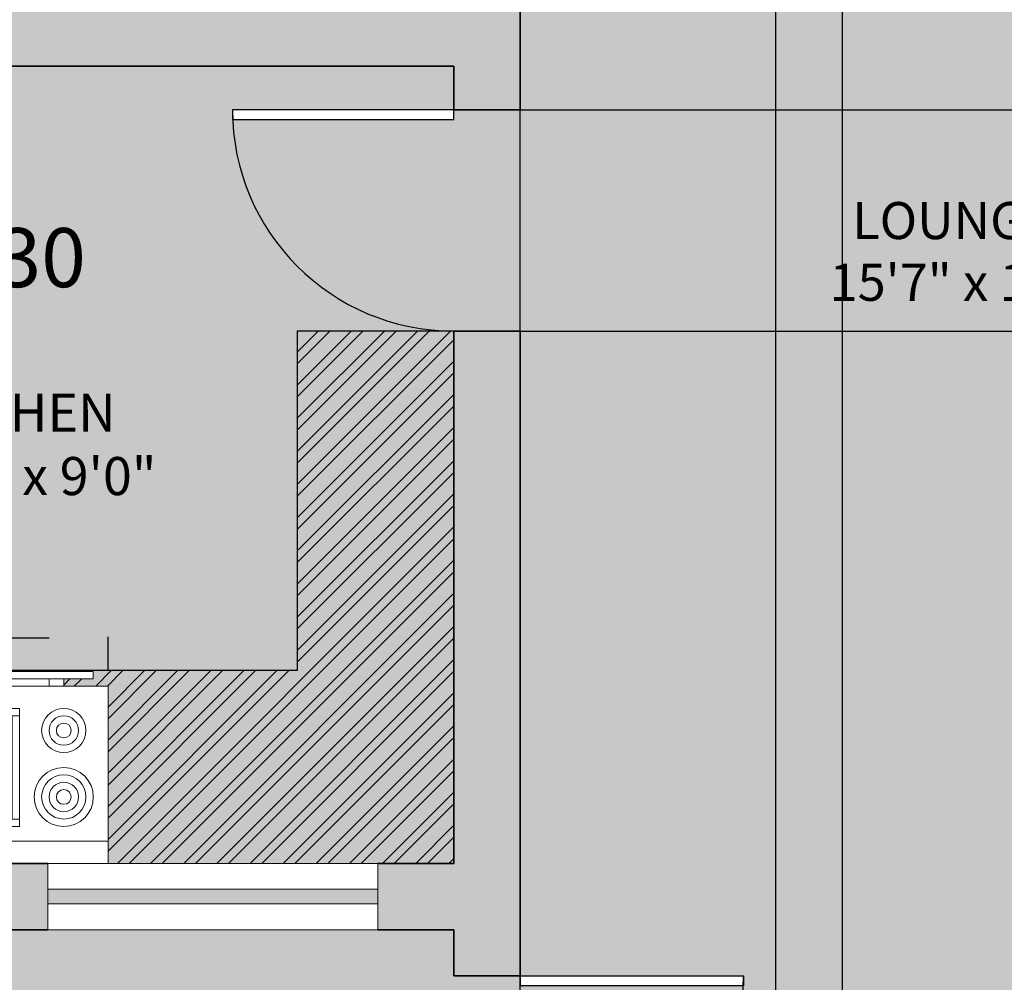
# Model space of a CAD drawing. Units: inches. Extents: x 389 to 971, y 148 to 870.
# Tile 9 of 14: x 537 to 670, y 428 to 558. Entities that reach past the tile are written whole.
import ezdxf

# ---------------------------------------------------------------- set-up
doc = ezdxf.new("R2010")
doc.units = ezdxf.units.IN
doc.header["$MEASUREMENT"] = 0
for name, color, linetype, lineweight in [('A-ANNO-DIMS', 2, 'Continuous', 18), ('A-AREA-IDEN', 7, 'Continuous', 18), ('A-CSWK-PATT', 9, 'Continuous', 13), ('A-DOOR', 4, 'Continuous', 25), ('A-EQPM', 8, 'Continuous', 18), ('A-FLOR-BASE-PATT', 8, 'Continuous', 13), ('A-FLOR-CSWK', 7, 'Continuous', 25), ('A-GLAZ', 4, 'Continuous', 18), ('A-WALL', 7, 'Continuous', 35), ('L-GRND-BASE-PATT', 8, 'Continuous', 13)]:
    doc.layers.add(name, color=color, linetype=linetype, lineweight=lineweight)
for name, color, linetype, lineweight, true_color in [('A-CSWK-BASE-PATT', 18, 'Continuous', 13, 0x000000), ('A-GLAZ-PATT', 251, 'Continuous', 13, 0x6d5f6c), ('A-WALL-PATT', 18, 'Continuous', 13, 0x000000), ('L-GRND-PATT', 39, 'Continuous', 13, 0x603913)]:
    doc.layers.add(name, color=color, linetype=linetype, lineweight=lineweight, true_color=true_color)
doc.styles.get("Standard").update_dxf_attribs({"font": 'arial.ttf'})
doc.dimstyles.get("Standard").update_dxf_attribs({"dimtxt": 8, "dimasz": 8, "dimexe": 0.18, "dimexo": 0.0625, "dimgap": 0.09, "dimtad": 0, "dimtih": 1, "dimtoh": 1, "dimdec": 0, "dimzin": 0, "dimdsep": 46, "dimlunit": 3, "dimtxsty": 'Standard', "dimcen": 0.09, "dimadec": 0, "dimazin": 0, "dimtfac": 1, "dimtdec": 0, "dimtofl": 0, "dimtmove": 0, "dimatfit": 3, "dimfxl": 1, "dimtolj": 1, "dimtzin": 0, "dimarcsym": 0})
pattern_1 = [(45, (0, 0), (-2.245064, 2.245064), []), (45, (0, 1.5875), (-2.245064, 2.245064), [])]

# ---------------------------------------------------------------- blocks, each defined once
blk = doc.blocks.new('*U2')
for p, q in [((0, 0), (0, -6)), ((40, 0), (40, -6))]:
    blk.add_line(p, q)
blk.add_lwpolyline([(0, 0), (0, 40), (1.75, 40), (1.75, 0)], close=True)
blk.add_arc((0, 0), 40, 0, 90)
blk = doc.blocks.new('*U3')
for p, q in [((0, 0), (0, -6)), ((-40, 0), (-40, -6))]:
    blk.add_line(p, q)
blk.add_lwpolyline([(0, 0), (0, 40), (-1.75, 40), (-1.75, 0)], close=True)
blk.add_arc((0, 0), 40, 90, 180)
blk = doc.blocks.new('Range-Oven - 30 in top')
for p, q in [((0, -3), (30, -3)), ((12, -6), (18, -6)), ((13, -20), (13, -6)), ((14, -6), (14, -20)), ((15, -20), (15, -6)), ((16, -6), (16, -20)), ((17, -20), (17, -6)), ((18, -20), (12, -20)), ((6, -24), (6, -25)), ((8, -25), (8, -24)), ((22, -25), (22, -24)), ((24, -24), (24, -25))]:
    blk.add_line(p, q)
for points in [[(0, -24), (0, 0), (30, 0), (30, -24)], [(12, -21), (12, -5), (18, -5), (18, -21)], [(2, -26), (2, -25), (28, -25), (28, -26)]]:
    blk.add_lwpolyline(points, close=True)
for centre, radius in [((6, -9), 4), ((6, -9), 3), ((24, -9), 3), ((6, -9), 2), ((6, -9), 1), ((24, -9), 2), ((24, -9), 1), ((24, -18), 4), ((6, -18), 3), ((6, -18), 2), ((24, -18), 3), ((24, -18), 2), ((6, -18), 1), ((24, -18), 1)]:
    blk.add_circle(centre, radius)
blk = doc.blocks.new('*D32')
at = {"layer": 'A-ANNO-DIMS', "color": 0, "lineweight": -2, "transparency": 16777216}
for p, q in [((518.55, 474.14), (510.55, 474.14)), ((518.55, 469.71), (518.55, 474.32)), ((540.55, 474.14), (526.55, 474.14)), ((548.55, 469.71), (548.55, 474.32))]:
    blk.add_line(p, q, dxfattribs=at)
at = {"layer": 'A-ANNO-DIMS', "color": 0, "transparency": 16777216}
for points in [[(526.55, 475.48), (526.55, 472.81), (518.55, 474.14)], [(540.55, 475.48), (540.55, 472.81), (548.55, 474.14)]]:
    blk.add_solid(points, dxfattribs=at)
at = {"layer": 'Defpoints', "color": 0, "transparency": 16777216}
for p in [(518.55, 474.14), (518.55, 469.64), (548.55, 469.64)]:
    blk.add_point(p, dxfattribs=at)
at = {"layer": 'A-ANNO-DIMS', "color": 0, "transparency": 16777216, "insert": (483.53, 474.14), "char_height": 8, "attachment_point": 5}
blk.add_mtext('\\A1;RANGE 30', dxfattribs=at)
blk = doc.blocks.new('*D34')
at = {"layer": 'A-ANNO-DIMS', "color": 0, "lineweight": -2, "transparency": 16777216}
for p, q in [((497.28, 540.7), (501.9, 540.7)), ((501.72, 532.7), (501.72, 529.93)), ((501.72, 518.7), (501.72, 521.47)), ((497.28, 510.7), (501.9, 510.7))]:
    blk.add_line(p, q, dxfattribs=at)
at = {"layer": 'A-ANNO-DIMS', "color": 0, "transparency": 16777216}
for points in [[(500.38, 532.7), (503.05, 532.7), (501.72, 540.7)], [(500.38, 518.7), (503.05, 518.7), (501.72, 510.7)]]:
    blk.add_solid(points, dxfattribs=at)
at = {"layer": 'Defpoints', "color": 0, "transparency": 16777216}
for p in [(497.22, 540.7), (501.72, 540.7), (497.22, 510.7)]:
    blk.add_point(p, dxfattribs=at)
at = {"layer": 'A-ANNO-DIMS', "color": 0, "transparency": 16777216, "insert": (501.72, 525.7), "char_height": 8, "attachment_point": 5}
blk.add_mtext('\\A1;KITCHEN SINK 30', dxfattribs=at)
blk = doc.blocks.new('*D48')
at = {"layer": 'A-ANNO-DIMS', "color": 0, "lineweight": -2, "transparency": 16777216}
for p, q in [((595.45, 545.73), (878.72, 545.73)), ((878.54, 537.73), (878.54, 534.91)), ((878.54, 523.73), (878.54, 526.55)), ((595.45, 515.73), (878.72, 515.73))]:
    blk.add_line(p, q, dxfattribs=at)
at = {"layer": 'A-ANNO-DIMS', "color": 0, "transparency": 16777216}
for points in [[(877.21, 537.73), (879.87, 537.73), (878.54, 545.73)], [(877.21, 523.73), (879.87, 523.73), (878.54, 515.73)]]:
    blk.add_solid(points, dxfattribs=at)
at = {"layer": 'Defpoints', "color": 0, "transparency": 16777216}
for p in [(595.39, 545.73), (878.54, 545.73), (595.39, 515.73)]:
    blk.add_point(p, dxfattribs=at)
at = {"layer": 'A-ANNO-DIMS', "color": 0, "transparency": 16777216, "insert": (878.54, 530.73), "char_height": 8, "attachment_point": 5}
blk.add_mtext('\\A1;30.005', dxfattribs=at)
blk = doc.blocks.new('*D51')
at = {"layer": 'A-ANNO-DIMS', "color": 0, "lineweight": -2, "transparency": 16777216}
for p, q in [((596.39, 864.97), (588.39, 864.97)), ((604.39, 354.78), (604.39, 865.15)), ((639.03, 354.78), (639.03, 865.15)), ((647.03, 864.97), (655.03, 864.97))]:
    blk.add_line(p, q, dxfattribs=at)
at = {"layer": 'A-ANNO-DIMS', "color": 0, "transparency": 16777216}
for points in [[(596.39, 866.3), (596.39, 863.64), (604.39, 864.97)], [(647.03, 866.3), (647.03, 863.64), (639.03, 864.97)]]:
    blk.add_solid(points, dxfattribs=at)
at = {"layer": 'Defpoints', "color": 0, "transparency": 16777216}
for p in [(639.03, 864.97), (604.39, 354.72), (639.03, 354.72)]:
    blk.add_point(p, dxfattribs=at)
at = {"layer": 'A-ANNO-DIMS', "color": 0, "transparency": 16777216, "insert": (621.71, 864.97), "char_height": 8, "attachment_point": 5}
blk.add_mtext('\\A1;34.64', dxfattribs=at)
blk = doc.blocks.new('*D52')
at = {"layer": 'A-ANNO-DIMS', "color": 0, "lineweight": -2, "transparency": 16777216}
for p, q in [((640.06, 864.97), (632.06, 864.97)), ((648.06, 388.98), (648.06, 865.15)), ((690.22, 388.98), (690.22, 865.15)), ((698.22, 864.97), (706.22, 864.97))]:
    blk.add_line(p, q, dxfattribs=at)
at = {"layer": 'A-ANNO-DIMS', "color": 0, "transparency": 16777216}
for points in [[(640.06, 866.3), (640.06, 863.64), (648.06, 864.97)], [(698.22, 866.3), (698.22, 863.64), (690.22, 864.97)]]:
    blk.add_solid(points, dxfattribs=at)
at = {"layer": 'Defpoints', "color": 0, "transparency": 16777216}
for p in [(690.22, 864.97), (648.06, 388.92), (690.22, 388.92)]:
    blk.add_point(p, dxfattribs=at)
at = {"layer": 'A-ANNO-DIMS', "color": 0, "transparency": 16777216, "insert": (669.14, 864.97), "char_height": 8, "attachment_point": 5}
blk.add_mtext('\\A1;42.155', dxfattribs=at)

msp = doc.modelspace()

# ---------------------------------------------------------------- hatches: boundary and pattern name
at = {"layer": 'A-CSWK-BASE-PATT'}
h = msp.add_hatch(color=256, dxfattribs=at)
h.dxf.hatch_style = 1
h.paths.add_polyline_path([(546.5523, 469.7503), (546.5523, 468.6445), (542.5523, 468.6445), (542.5523, 467.6445), (548.5523, 467.6445), (548.5523, 443.6445), (585.0791, 443.6445), (595.387, 443.6445), (595.387, 515.7271), (574.1873, 515.7271), (574.1873, 469.7503)])
at = {"layer": 'A-CSWK-PATT'}
h = msp.add_hatch(dxfattribs=at)
h.set_pattern_fill('STEEL', color=256)
h.set_pattern_definition(pattern_1)
h.paths.add_polyline_path([(477.216, 551.6445), (477.216, 543.0462), (477.216, 508.3496), (477.216, 490.1255), (477.216, 452.1978), (477.216, 443.6445), (488.4095, 443.6445), (526.7125, 443.6445), (540.3922, 443.6445), (585.0791, 443.6445), (595.387, 443.6445), (595.387, 515.7271), (574.1873, 515.7271), (574.1873, 469.7503), (497.3577, 469.7503), (497.3577, 551.6445)])
h.paths.add_polyline_path([(495.716, 540.6979, -0.41421356), (497.216, 539.1979), (497.216, 512.1979, -0.41421356), (495.716, 510.6979), (478.716, 510.6979, -0.41421356), (477.216, 512.1979), (477.216, 539.1979, -0.41421356), (478.716, 540.6979)], flags=0)
h.paths.add_polyline_path([(494.716, 539.1979, -0.41421356), (495.716, 538.1979), (495.716, 513.1979, -0.41421356), (494.716, 512.1979), (483.716, 512.1979, -0.41421356), (482.716, 513.1979), (482.716, 538.1979, -0.41421356), (483.716, 539.1979)], flags=16)
h.paths.add_polyline_path([(490.216, 525.6979, -1), (488.216, 525.6979, -1)], flags=0)
h.paths.add_polyline_path([(489.716, 525.6979, -1), (488.716, 525.6979, -1)], flags=0)
h.paths.add_polyline_path([(520.5523, 469.6445), (546.5523, 469.6445), (546.5523, 468.6445), (542.5523, 468.6445), (542.5523, 467.6445), (548.5523, 467.6445), (548.5523, 443.6445), (518.5523, 443.6445), (518.5523, 467.6445), (524.5523, 467.6445), (524.5523, 468.6445), (520.5523, 468.6445)], flags=16)
h.paths.add_polyline_path([(528.5523, 461.6445, -1), (520.5523, 461.6445, -1)], flags=0)
h.paths.add_polyline_path([(527.5523, 461.6445, -1), (521.5523, 461.6445, -1)], flags=0)
h.paths.add_polyline_path([(526.5523, 461.6445, -1), (522.5523, 461.6445, -1)], flags=0)
h.paths.add_polyline_path([(525.5523, 461.6445, -1), (523.5523, 461.6445, -1)], flags=0)
h.paths.add_polyline_path([(530.5523, 464.6445), (536.5523, 464.6445), (536.5523, 448.6445), (530.5523, 448.6445)], flags=0)
h.paths.add_polyline_path([(535.5523, 463.6445), (535.5523, 449.6445), (531.5523, 449.6445), (531.5523, 463.6445)], flags=0)
h.paths.add_polyline_path([(527.5523, 452.6445, -1), (521.5523, 452.6445, -1)], flags=0)
h.paths.add_polyline_path([(545.5523, 461.6445, -1), (539.5523, 461.6445, -1)], flags=0)
h.paths.add_polyline_path([(526.5523, 452.6445, -1), (522.5523, 452.6445, -1)], flags=0)
h.paths.add_polyline_path([(544.5523, 461.6445, -1), (540.5523, 461.6445, -1)], flags=0)
h.paths.add_polyline_path([(525.5523, 452.6445, -1), (523.5523, 452.6445, -1)], flags=0)
h.paths.add_polyline_path([(543.5523, 461.6445, -1), (541.5523, 461.6445, -1)], flags=0)
h.paths.add_polyline_path([(546.5523, 452.6445, -1), (538.5523, 452.6445, -1)], flags=0)
h.paths.add_polyline_path([(545.5523, 452.6445, -1), (539.5523, 452.6445, -1)], flags=0)
h.paths.add_polyline_path([(544.5523, 452.6445, -1), (540.5523, 452.6445, -1)], flags=0)
h.paths.add_polyline_path([(543.5523, 452.6445, -1), (541.5523, 452.6445, -1)], flags=0)
h = msp.add_hatch(dxfattribs=at)
h.set_pattern_fill('STEEL', color=256)
h.set_pattern_definition(pattern_1)
h.paths.add_polyline_path([(595.387, 515.7271), (574.1873, 515.7271), (574.1873, 469.7503), (546.5523, 469.7503), (546.5523, 468.6445), (542.5523, 468.6445), (542.5523, 467.6445), (548.5523, 467.6445), (548.5523, 443.6445), (585.0791, 443.6445), (595.387, 443.6445)])
at = {"layer": 'A-FLOR-BASE-PATT'}
h = msp.add_hatch(color=256, dxfattribs=at)
h.dxf.hatch_style = 1
h.paths.add_polyline_path([(634.6594, 428.4021), (634.6594, 427.0792), (634.6305, 427.0792, -0.40145271), (604.4225, 398.1652), (604.0817, 398.1199, -0.40145271), (632.0195, 371.3788), (632.0462, 371.3788), (632.0462, 370.1554), (604.387, 370.1554), (604.387, 366.7191), (640.0296, 366.7191), (640.0296, 321.4969, 1), (647.061, 321.4969), (647.061, 412.9189), (690.216, 412.9189), (690.216, 416.0006), (694.716, 416.0006), (702.2145, 416.0006, 0.39601219), (737.1392, 448.8066), (702.2145, 448.8066), (702.2145, 450.9936), (694.716, 450.9936), (690.216, 450.9936), (690.216, 466.6012), (708.7881, 466.6012), (708.7881, 462.1012), (784.6145, 462.1012), (784.6145, 466.6012), (794.216, 466.6012), (794.216, 591.6445), (708.5171, 591.6445), (708.5171, 596.1445), (708.5171, 602.9755, 0.39601219), (678.6314, 634.7912), (678.6314, 602.9755), (676.6391, 602.9755), (676.6391, 596.1445), (676.6391, 591.6445), (661.216, 591.6445), (661.216, 632.6445), (653.109, 632.6445), (653.109, 641.6445), (653.109, 642.1751), (651.6417, 642.1751), (651.6417, 675.6801, 0.40145271), (619.5719, 642.1751), (619.5719, 637.1445), (619.5147, 632.6445), (604.387, 632.6445), (604.387, 545.7317), (595.3894, 545.7317), (595.3894, 544.4199), (565.4338, 544.4199, 0.40145271), (595.3894, 515.7475), (599.887, 515.7475), (604.387, 515.7271), (604.387, 428.4021)])
h.paths.add_polyline_path([(721.8003, 493.9292), (725.0899, 493.9292), (725.0899, 493.075), (751.4065, 493.075), (751.4065, 493.9292), (754.6961, 493.9292), (754.6961, 479.6744, -0.26666697), (721.8003, 479.6744)], flags=16)
h.paths.add_polyline_path([(720.6421, 516.0583), (720.6421, 545.0393), (753.5806, 545.0393), (753.5806, 516.0583)], flags=16)
h.paths.add_polyline_path([(722.6421, 518.0583), (722.6421, 543.0393), (751.5806, 543.0393), (751.5806, 518.0583)], flags=0)
h.paths.add_polyline_path([(763.7396, 488.5801), (763.7822, 488.1156), (764.1436, 488.1761)], flags=16)
h.paths.add_polyline_path([(777.9011, 479.7417), (778.0475, 480.1886), (777.4745, 480.275)], flags=16)
h.paths.add_polyline_path([(762.3329, 503.5919), (762.3329, 507.1718), (763.2624, 507.1718), (763.2624, 550.1306), (762.3329, 550.1306), (762.3329, 553.7105), (777.8458, 553.7105, -0.19047621), (777.8458, 503.5919)], flags=16)
h.paths.add_polyline_path([(721.6097, 567.2898), (721.6097, 581.7362, -0.26666697), (754.9475, 581.7362), (754.9475, 567.2898), (751.6137, 567.2898), (751.6137, 568.1555), (724.9435, 568.1555), (724.9435, 567.2898)], flags=16)
h.paths.add_polyline_path([(774.6347, 521.4914), (774.6347, 535.811), (778.6837, 535.811, -0.04962821), (778.6837, 521.4914)], flags=0)
h.paths.add_polyline_path([(764.6624, 576.8996), (764.7454, 576.4742), (765.0717, 576.4903)], flags=16)
h.paths.add_polyline_path([(777.2772, 570.3652), (777.4444, 570.8756), (776.7899, 570.9743)], flags=16)
h.paths.add_polyline_path([(644.2892, 516.9956), (685.2491, 516.9956), (685.2491, 535.7223), (644.2892, 535.7223)], flags=24)
h = msp.add_hatch(color=256, dxfattribs=at)
h.dxf.hatch_style = 1
h.paths.add_polyline_path([(497.3577, 469.7503), (574.1873, 469.7503), (574.1873, 515.7271), (595.387, 515.7271), (595.5252, 515.7478, -0.40276815), (565.4338, 544.4199), (565.4051, 544.4199), (565.4051, 545.7317), (595.387, 545.7317), (595.387, 551.6445), (497.3577, 551.6445)])
h.paths.add_polyline_path([(516.2555, 490.6064), (554.3542, 490.6064), (554.3542, 509.8575), (516.2555, 509.8575)], flags=24)
at = {"layer": 'A-GLAZ-PATT'}
h = msp.add_hatch(color=256, dxfattribs=at)
h.dxf.hatch_style = 1
h.paths.add_polyline_path([(540.3922, 440.1445), (540.3922, 438.1445), (585.0791, 438.1445), (585.0791, 440.1445)])
at = {"layer": 'A-WALL-PATT'}
h = msp.add_hatch(color=256, dxfattribs=at)
h.dxf.hatch_style = 1
h.paths.add_polyline_path([(538.3237, 641.6445), (538.3237, 637.1445), (538.3237, 632.6445), (595.387, 632.6445), (595.387, 560.6445), (558.5088, 560.6445), (511.387, 560.6445), (511.387, 585.4344), (502.387, 585.4344), (502.387, 560.6445), (468.216, 560.6445), (468.216, 543.0462), (477.216, 543.0462), (477.216, 551.6445), (595.387, 551.6445), (595.387, 545.7317), (595.3894, 545.7317), (599.887, 545.7317), (604.387, 545.7317), (604.387, 632.6445), (619.5147, 632.6445), (619.5147, 641.6445)])
h = msp.add_hatch(color=256, dxfattribs=at)
h.dxf.hatch_style = 1
h.paths.add_polyline_path([(595.387, 443.6445), (585.0791, 443.6445), (585.0791, 434.6445), (595.387, 434.6445), (595.387, 428.4021), (604.387, 428.4021), (604.387, 515.7271), (595.387, 515.7271)])
h = msp.add_hatch(color=256, dxfattribs=at)
h.dxf.hatch_style = 1
h.paths.add_polyline_path([(540.3922, 434.6445), (540.3922, 443.6445), (526.7125, 443.6445), (526.7125, 434.6445)])
at = {"layer": 'L-GRND-BASE-PATT'}
h = msp.add_hatch(color=256, dxfattribs=at)
h.dxf.hatch_style = 1
edge = h.paths.add_edge_path(flags=16)
edge.add_ellipse((8782.0026, 354.2473), major_axis=(-8296.9493, 0), ratio=0.84230387, start_angle=-0.09022909, end_angle=0.38386678, ccw=False)
edge.add_ellipse((485.0533, 368.2895), major_axis=(-1.1591, 0), ratio=0.84230387, start_angle=0, end_angle=90, ccw=False)
edge.add_line((483.8943, 368.2895), (483.8943, 387.6039))
edge.add_ellipse((485.0533, 387.2466), major_axis=(1.1591, 0), ratio=0.84230387, start_angle=90, end_angle=180, ccw=False)
edge.add_line((485.0533, 388.2229), (485.5047, 388.2229))
edge.add_ellipse((898.8202, 372.4897), major_axis=(413.7374, 0), ratio=0.84230387, start_angle=176.349572, end_angle=177.82005, ccw=False)
edge.add_ellipse((535.9119, 196.3855), major_axis=(-245.3972, 0), ratio=0.84230387, start_angle=-77.874034, end_angle=-76.219471, ccw=False)
edge.add_ellipse((535.9119, 201.7547), major_axis=(239.1274, 0), ratio=0.84230387, start_angle=100.209539, end_angle=102.444627, ccw=False)
edge.add_ellipse((473.3139, 564.9222), major_axis=(196.5637, 0), ratio=0.84230387, start_angle=-80.743434, end_angle=-77.445067)
edge.add_line((509.5535, 402.1941), (514.3535, 404.8483))
edge.add_line((514.3535, 404.8483), (514.3535, 404.7972))
edge.add_ellipse((514.3535, 404.2644), major_axis=(0.5795, 0), ratio=0.84230387, start_angle=52.06687, end_angle=90, ccw=False)
edge.add_line((514.6716, 404.6725), (519.1535, 402.1941))
edge.add_ellipse((555.3932, 564.9222), major_axis=(-196.5637, 0), ratio=0.84230387, start_angle=77.445067, end_angle=80.743434)
edge.add_ellipse((492.7951, 201.7547), major_axis=(239.1274, 0), ratio=0.84230387, start_angle=77.555373, end_angle=79.790461, ccw=False)
edge.add_ellipse((492.7951, 196.3855), major_axis=(245.3972, 0), ratio=0.84230387, start_angle=76.219471, end_angle=77.874034, ccw=False)
edge.add_ellipse((129.8868, 372.4897), major_axis=(-413.7374, 0), ratio=0.84230387, start_angle=182.17995, end_angle=183.650428, ccw=False)
edge.add_line((543.2023, 388.2229), (544.0779, 388.2229))
edge.add_ellipse((543.6537, 387.2466), major_axis=(-1.1591, 0), ratio=0.84230387, start_angle=180, end_angle=270, ccw=False)
edge.add_line((544.8128, 387.2466), (544.8128, 367.9322))
edge.add_ellipse((543.6537, 368.2895), major_axis=(1.1591, 0), ratio=0.84230387, start_angle=270, end_angle=360, ccw=False)
edge.add_ellipse((-7753.2956, 354.2473), major_axis=(-8296.9493, 0), ratio=0.84230387, start_angle=179.61613322, end_angle=180.09022909, ccw=False)
edge.add_line((543.3912, 298.6608), (544.0779, 298.6608))
edge.add_ellipse((543.6537, 297.6845), major_axis=(1.1591, 0), ratio=0.84230387, start_angle=0, end_angle=90, ccw=False)
edge.add_line((544.8128, 297.6845), (544.8128, 278.3701))
edge.add_ellipse((543.6537, 278.7275), major_axis=(-1.1591, 0), ratio=0.84230387, start_angle=90, end_angle=180, ccw=False)
edge.add_line((543.6537, 277.7512), (543.1566, 277.7512))
edge.add_ellipse((-7753.2956, 354.2473), major_axis=(-8296.9493, 0), ratio=0.84230387, start_angle=179.3813568, end_angle=179.47172853, ccw=False)
edge.add_ellipse((542.4236, 263.2763), major_axis=(-1.7386, 0), ratio=0.84230387, start_angle=179.371763, end_angle=248.464757, ccw=False)
edge.add_ellipse((-7753.8751, 354.2473), major_axis=(-8298.7403, 0), ratio=0.842303866, start_angle=179.35344592, end_angle=179.3717628, ccw=False)
edge.add_ellipse((540.0116, 260.6509), major_axis=(-4.1092, 0), ratio=0.84230387, start_angle=90, end_angle=179.353446, ccw=False)
edge.add_line((540.0116, 257.1897), (488.6954, 257.1897))
edge.add_ellipse((488.6954, 260.6509), major_axis=(4.1092, 0), ratio=0.84230387, start_angle=180.646554, end_angle=270, ccw=False)
edge.add_ellipse((8782.5821, 354.2473), major_axis=(-8298.7403, 0), ratio=0.842303872, start_angle=0.62823723, end_angle=0.64655411, ccw=False)
edge.add_ellipse((486.2834, 263.2763), major_axis=(-1.7386, 0), ratio=0.84230387, start_angle=-68.464756, end_angle=0.628237, ccw=False)
edge.add_ellipse((8782.0026, 354.2473), major_axis=(-8296.9493, 0), ratio=0.84230387, start_angle=0.52827147, end_angle=0.6465541, ccw=False)
edge.add_line((485.5504, 277.7512), (484.6291, 277.7512))
edge.add_ellipse((485.0533, 278.7275), major_axis=(-1.1591, 0), ratio=0.84230387, start_angle=0, end_angle=90, ccw=False)
edge.add_line((483.8943, 278.7275), (483.8943, 298.0418))
edge.add_ellipse((485.0533, 297.6845), major_axis=(1.1591, 0), ratio=0.84230387, start_angle=90, end_angle=180, ccw=False)
edge = h.paths.add_edge_path(flags=0)
edge.add_ellipse((8782.0026, 354.2473), major_axis=(-8295.7902, 0), ratio=0.84230387, start_angle=0.05559431, end_angle=0.37776419, ccw=False)
edge.add_line((486.2179, 346.1978), (489.3905, 335.8384))
edge.add_ellipse((3386.0114, 329.7263), major_axis=(-2896.63, 0), ratio=0.84230387, start_angle=-0.1208974, end_angle=0.3640763)
edge.add_line((489.4638, 311.3204), (486.4666, 299.5521))
edge = h.paths.add_edge_path(flags=0)
edge.add_ellipse((514.3535, 391.3731), major_axis=(-115.1513, 0), ratio=0.84230387, start_angle=76.401865, end_angle=103.598135)
edge.add_line((537.3428, 296.3333), (537.3428, 281.5897))
edge.add_ellipse((514.3535, 376.6295), major_axis=(-115.1513, 0), ratio=0.84230387, start_angle=76.401865, end_angle=103.598135, ccw=False)
edge.add_line((491.3643, 281.5897), (491.3643, 296.3333))
edge = h.paths.add_edge_path(flags=0)
edge.add_line((491.3643, 337.0752), (489.653, 349.9016))
edge.add_ellipse((510.1338, 298.7862), major_axis=(64.0481, 0), ratio=0.84230387, start_angle=94.277421, end_angle=111.834954, ccw=False)
edge.add_line((506.1068, 352.6274), (522.6002, 352.6274))
edge.add_ellipse((518.5732, 298.7862), major_axis=(64.0481, 0), ratio=0.84230387, start_angle=68.165046, end_angle=85.722579, ccw=False)
edge.add_line((539.0541, 349.9016), (537.3428, 337.0752))
edge.add_ellipse((516.5462, 287.5825), major_axis=(62.3305, 0), ratio=0.84230387, start_angle=67.208085, end_angle=85.12993)
edge.add_line((521.008, 339.949), (507.699, 339.949))
edge.add_ellipse((512.1609, 287.5825), major_axis=(62.3305, 0), ratio=0.84230387, start_angle=94.87007, end_angle=112.791915)
edge = h.paths.add_edge_path(flags=0)
edge.add_ellipse((493.6824, 273.9439), major_axis=(-2.3182, 0), ratio=0.84230387, start_angle=-90, end_angle=0, ccw=False)
edge.add_line((493.6824, 275.8965), (535.3743, 275.8965))
edge.add_ellipse((535.0246, 273.9439), major_axis=(2.3182, 0), ratio=0.84230387, start_angle=0, end_angle=90, ccw=False)
edge.add_line((537.3428, 273.9439), (537.3428, 258.6983))
edge.add_line((537.3428, 258.6983), (540.5912, 258.6983))
edge.add_ellipse((540.5912, 260.6509), major_axis=(-2.3182, 0), ratio=0.84230387, start_angle=90, end_angle=179.353446)
edge.add_line((540.5912, 258.6983), (487.7691, 258.6983))
edge.add_ellipse((488.1158, 260.6509), major_axis=(2.3182, 0), ratio=0.84230387, start_angle=180.646554, end_angle=270)
edge.add_line((488.1158, 258.6983), (491.3643, 258.6983))
edge.add_line((491.3643, 258.6983), (491.3643, 274.2384))
h.paths.add_polyline_path([(746.1376, 327.3223), (750.14, 327.3223), (750.14, 326.2831), (798.1694, 326.2831), (798.1694, 327.3223), (802.1718, 327.3223), (802.1718, 309.9784, -0.19047621), (746.1376, 309.9784)], flags=16)
h.paths.add_polyline_path([(782.1596, 313.5685), (782.1596, 309.0415, -0.04962821), (766.1498, 309.0415), (766.1498, 313.5685)], flags=0)
h.paths.add_polyline_path([(755.1859, 344.9352), (755.1859, 373.9163), (788.1244, 373.9163), (788.1244, 344.9352)], flags=16)
h.paths.add_polyline_path([(757.1859, 346.9352), (757.1859, 371.9163), (786.1244, 371.9163), (786.1244, 346.9352)], flags=0)
h.paths.add_polyline_path([(803.6446, 338.4879), (803.6446, 342.4903), (804.6838, 342.4903), (804.6838, 390.5197), (803.6446, 390.5197), (803.6446, 394.5221), (820.9885, 394.5221, -0.19047621), (820.9885, 338.4879)], flags=16)
h.paths.add_polyline_path([(806.8707, 326.6963), (806.4254, 327.1416), (806.4724, 326.6297)], flags=16)
h.paths.add_polyline_path([(822.0328, 317.4008), (822.1942, 317.8933), (821.5626, 317.9885)], flags=16)
h.paths.add_polyline_path([(817.3984, 358.5001), (817.3984, 374.5099), (821.9254, 374.5099, -0.04962821), (821.9254, 358.5001)], flags=0)
h.paths.add_polyline_path([(808.1446, 418.9737), (808.2247, 418.5632), (808.5395, 418.5787)], flags=16)
h.paths.add_polyline_path([(820.3159, 412.669), (820.4772, 413.1615), (819.8457, 413.2568)], flags=16)
h.paths.add_polyline_path([(466.3155, 235.5246), (517.3807, 235.5246), (517.3807, 244.4269), (466.3155, 244.4269)], flags=24)
h.paths.add_polyline_path([(739.8737, 256.2), (815.404, 256.2), (815.404, 265.3454), (739.8737, 265.3454)], flags=24)
h.paths.add_polyline_path([(750.6082, 393.6667), (791.5681, 393.6667), (791.5681, 412.3933), (750.6082, 412.3933)], flags=24)
h.paths.add_polyline_path([(438.9631, 410.0619), (484.6204, 410.0619), (484.6204, 429.1217), (438.9631, 429.1217)], flags=24)
edge = h.paths.add_edge_path()
edge.add_line((839.216, 285.6445), (611.8787, 285.6445))
edge.add_line((611.8787, 285.6445), (604.387, 285.6445))
edge.add_line((604.387, 285.6445), (595.387, 285.6445))
edge.add_line((595.387, 285.6445), (595.387, 370.1554))
edge.add_line((595.387, 370.1554), (604.0817, 370.1554))
edge.add_line((604.0817, 370.1554), (604.0817, 371.3788))
edge.add_line((604.0817, 371.3788), (632.0195, 371.3788))
edge.add_arc((604.0817, 370.1554), 27.9645, 2.507491, 90)
edge.add_line((604.0817, 398.1199), (599.887, 398.1652))
edge.add_line((599.887, 398.1652), (604.4225, 398.1652))
edge.add_arc((604.4225, 428.4021), 30.2369, 270, 357.492509)
edge.add_line((634.6305, 427.0792), (604.4225, 427.0792))
edge.add_line((604.4225, 427.0792), (604.4225, 428.4021))
edge.add_line((604.4225, 428.4021), (599.887, 428.4021))
edge.add_line((599.887, 428.4021), (595.387, 428.4021))
edge.add_line((595.387, 428.4021), (595.387, 434.6445))
edge.add_line((595.387, 434.6445), (585.0791, 434.6445))
edge.add_line((585.0791, 434.6445), (540.3922, 434.6445))
edge.add_line((540.3922, 434.6445), (526.7125, 434.6445))
edge.add_line((526.7125, 434.6445), (488.4095, 434.6445))
edge.add_line((488.4095, 434.6445), (432.216, 434.6445))
edge.add_line((432.216, 434.6445), (432.216, 243.6445))
edge.add_line((432.216, 243.6445), (437.216, 243.6445))
edge.add_line((437.216, 243.6445), (437.216, 234.6445))
edge.add_line((437.216, 234.6445), (581.216, 234.6445))
edge.add_line((581.216, 234.6445), (581.216, 238.6445))
edge.add_line((581.216, 238.6445), (581.216, 243.6445))
edge.add_line((581.216, 243.6445), (590.216, 243.6445))
edge.add_line((590.216, 243.6445), (590.216, 238.6445))
edge.add_line((590.216, 238.6445), (839.216, 238.6445))
edge.add_line((839.216, 238.6445), (839.216, 285.6445))
at = {"layer": 'L-GRND-PATT'}
h = msp.add_hatch(dxfattribs=at)
h.set_pattern_fill('EARTH', color=256, angle=45)
h.set_pattern_definition([(45, (0, 0), (0, 8.980256), [6.35, -6.35]), (45, (-1.684, 1.684), (0, 8.980256), [6.35, -6.35]), (45, (-3.3676, 3.3676), (0, 8.980256), [6.35, -6.35]), (135, (-3.3676, 4.49), (-8.980256, 0), [6.35, -6.35]), (135, (-1.684, 6.174), (-8.980256, 0), [6.35, -6.35]), (135, (0, 7.858), (-8.980256, 0), [6.35, -6.35])])
h.paths.add_polyline_path([(432.216, 243.6445), (437.216, 243.6445), (437.216, 234.6445), (581.216, 234.6445), (581.216, 238.6445), (581.216, 243.6445), (590.216, 243.6445), (590.216, 238.6445), (839.216, 238.6445), (839.216, 285.6445), (810.0514, 285.6445), (733.8057, 285.6445), (684.2434, 285.6445), (611.8787, 285.6445), (604.387, 285.6445), (595.387, 285.6445), (595.387, 370.1554), (604.0817, 370.1554), (604.0817, 371.3788), (632.0195, 371.3788, 0.40145271), (604.0817, 398.1199), (599.887, 398.1652), (604.4225, 398.1652, 0.40145271), (634.6305, 427.0792), (604.4225, 427.0792), (604.4225, 428.4021), (599.887, 428.4021), (595.387, 428.4021), (595.387, 434.6445), (585.0791, 434.6445), (540.3922, 434.6445), (526.7125, 434.6445), (488.4095, 434.6445), (432.216, 434.6445)])
edge = h.paths.add_edge_path(flags=16)
edge.add_line((483.8943, 278.7275), (483.8943, 298.2564))
edge.add_ellipse((485.0533, 297.6845), major_axis=(1.1591, 0), ratio=0.84230387, start_angle=90, end_angle=180, ccw=False)
edge.add_ellipse((8782.0026, 354.2473), major_axis=(-8296.9493, 0), ratio=0.84230387, start_angle=-0.09022909, end_angle=0.38386678, ccw=False)
edge.add_ellipse((485.0533, 368.2895), major_axis=(-1.1591, 0), ratio=0.84230387, start_angle=0, end_angle=90, ccw=False)
edge.add_line((483.8943, 368.2895), (483.8943, 387.8185))
edge.add_ellipse((485.0533, 387.2466), major_axis=(1.1591, 0), ratio=0.84230387, start_angle=90, end_angle=180, ccw=False)
edge.add_ellipse((898.8202, 372.4897), major_axis=(413.7374, 0), ratio=0.84230387, start_angle=176.349572, end_angle=177.82005, ccw=False)
edge.add_ellipse((535.9119, 196.3855), major_axis=(-245.3972, 0), ratio=0.84230387, start_angle=-77.874034, end_angle=-76.219471, ccw=False)
edge.add_ellipse((535.9119, 201.7547), major_axis=(239.1274, 0), ratio=0.84230387, start_angle=100.209539, end_angle=102.444627, ccw=False)
edge.add_ellipse((473.3139, 564.9222), major_axis=(196.5637, 0), ratio=0.84230387, start_angle=-80.743434, end_angle=-77.445067)
edge.add_line((509.5535, 402.1941), (514.3535, 404.8483))
edge.add_line((514.3535, 404.8483), (519.1535, 402.1941))
edge.add_ellipse((555.3932, 564.9222), major_axis=(-196.5637, 0), ratio=0.84230387, start_angle=77.445067, end_angle=80.743434)
edge.add_ellipse((492.7951, 201.7547), major_axis=(239.1274, 0), ratio=0.84230387, start_angle=77.555373, end_angle=79.790461, ccw=False)
edge.add_ellipse((492.7951, 196.3855), major_axis=(245.3972, 0), ratio=0.84230387, start_angle=76.219471, end_angle=77.874034, ccw=False)
edge.add_ellipse((129.8868, 372.4897), major_axis=(-413.7374, 0), ratio=0.84230387, start_angle=182.17995, end_angle=183.650428, ccw=False)
edge.add_line((543.2023, 388.2229), (544.3327, 388.2229))
edge.add_ellipse((543.6537, 387.2466), major_axis=(-1.1591, 0), ratio=0.84230387, start_angle=180, end_angle=270, ccw=False)
edge.add_line((544.8128, 387.2466), (544.8128, 367.7176))
edge.add_ellipse((543.6537, 368.2895), major_axis=(1.1591, 0), ratio=0.84230387, start_angle=270, end_angle=360, ccw=False)
edge.add_ellipse((-7753.2956, 354.2473), major_axis=(-8296.9493, 0), ratio=0.84230387, start_angle=179.61613322, end_angle=180.09022909, ccw=False)
edge.add_ellipse((543.6537, 297.6845), major_axis=(1.1591, 0), ratio=0.84230387, start_angle=0, end_angle=90, ccw=False)
edge.add_line((544.8128, 297.6845), (544.8128, 278.1556))
edge.add_ellipse((543.6537, 278.7275), major_axis=(-1.1591, 0), ratio=0.84230387, start_angle=90, end_angle=180, ccw=False)
edge.add_ellipse((-7753.2956, 354.2473), major_axis=(-8296.9493, 0), ratio=0.84230387, start_angle=179.3813568, end_angle=179.47172853, ccw=False)
edge.add_ellipse((542.4236, 263.2763), major_axis=(-1.7386, 0), ratio=0.84230387, start_angle=179.371763, end_angle=248.464757, ccw=False)
edge.add_ellipse((-7753.8751, 354.2473), major_axis=(-8298.7403, 0), ratio=0.842303866, start_angle=179.35344592, end_angle=179.3717628, ccw=False)
edge.add_ellipse((540.0116, 260.6509), major_axis=(-4.1092, 0), ratio=0.84230387, start_angle=90, end_angle=179.353446, ccw=False)
edge.add_line((540.0116, 257.1897), (488.0808, 257.1897))
edge.add_ellipse((488.6954, 260.6509), major_axis=(4.1092, 0), ratio=0.84230387, start_angle=180.646554, end_angle=270, ccw=False)
edge.add_ellipse((8782.5821, 354.2473), major_axis=(-8298.7403, 0), ratio=0.842303872, start_angle=0.62823723, end_angle=0.64655411, ccw=False)
edge.add_ellipse((486.2834, 263.2763), major_axis=(-1.7386, 0), ratio=0.84230387, start_angle=-68.464756, end_angle=0.628237, ccw=False)
edge.add_ellipse((8782.0026, 354.2473), major_axis=(-8296.9493, 0), ratio=0.84230387, start_angle=0.52827147, end_angle=0.6465541, ccw=False)
edge.add_line((485.5504, 277.7512), (484.3744, 277.7512))
edge.add_ellipse((485.0533, 278.7275), major_axis=(-1.1591, 0), ratio=0.84230387, start_angle=0, end_angle=90, ccw=False)
edge = h.paths.add_edge_path(flags=0)
edge.add_ellipse((488.1158, 260.6509), major_axis=(2.3182, 0), ratio=0.84230387, start_angle=180.646554, end_angle=270)
edge.add_line((488.1158, 258.6983), (491.3643, 258.6983))
edge.add_line((491.3643, 258.6983), (491.3643, 274.4686))
edge.add_ellipse((493.6824, 273.9439), major_axis=(-2.3182, 0), ratio=0.84230387, start_angle=-90, end_angle=0, ccw=False)
edge.add_line((493.6824, 275.8965), (535.6476, 275.8965))
edge.add_ellipse((535.0246, 273.9439), major_axis=(2.3182, 0), ratio=0.84230387, start_angle=0, end_angle=90, ccw=False)
edge.add_line((537.3428, 273.9439), (537.3428, 258.6983))
edge.add_line((537.3428, 258.6983), (541.2086, 258.6983))
edge.add_ellipse((540.5912, 260.6509), major_axis=(-2.3182, 0), ratio=0.84230387, start_angle=90, end_angle=179.353446, ccw=False)
edge.add_line((540.5912, 258.6983), (487.4984, 258.6983))
edge = h.paths.add_edge_path(flags=0)
edge.add_line((491.3643, 281.5897), (491.3643, 296.3333))
edge.add_ellipse((514.3535, 391.3731), major_axis=(-115.1513, 0), ratio=0.84230387, start_angle=76.401865, end_angle=103.598135)
edge.add_line((537.3428, 296.3333), (537.3428, 281.5897))
edge.add_ellipse((514.3535, 376.6295), major_axis=(-115.1513, 0), ratio=0.84230387, start_angle=76.401865, end_angle=103.598135, ccw=False)
edge = h.paths.add_edge_path(flags=0)
edge.add_ellipse((8782.0026, 354.2473), major_axis=(-8295.7902, 0), ratio=0.84230387, start_angle=0.05559431, end_angle=0.37776419, ccw=False)
edge.add_line((486.2179, 346.1978), (489.3905, 335.8384))
edge.add_ellipse((3386.0114, 329.7263), major_axis=(-2896.63, 0), ratio=0.84230387, start_angle=-0.1208974, end_angle=0.3640763)
edge.add_line((489.4638, 311.3204), (486.4666, 299.5521))
edge = h.paths.add_edge_path(flags=0)
edge.add_line((491.3643, 337.0752), (489.653, 349.9016))
edge.add_ellipse((510.1338, 298.7862), major_axis=(64.0481, 0), ratio=0.84230387, start_angle=94.277421, end_angle=111.834954, ccw=False)
edge.add_line((506.1068, 352.6274), (522.6002, 352.6274))
edge.add_ellipse((518.5732, 298.7862), major_axis=(64.0481, 0), ratio=0.84230387, start_angle=68.165046, end_angle=85.722579, ccw=False)
edge.add_line((539.0541, 349.9016), (537.3428, 337.0752))
edge.add_ellipse((516.5462, 287.5825), major_axis=(62.3305, 0), ratio=0.84230387, start_angle=67.208085, end_angle=85.12993)
edge.add_line((521.008, 339.949), (507.699, 339.949))
edge.add_ellipse((512.1609, 287.5825), major_axis=(62.3305, 0), ratio=0.84230387, start_angle=94.87007, end_angle=112.791915)
h.paths.add_polyline_path([(466.3155, 235.5246), (517.3807, 235.5246), (517.3807, 244.4269), (466.3155, 244.4269)], flags=24)
h.paths.add_polyline_path([(739.8737, 256.2), (815.404, 256.2), (815.404, 265.3454), (739.8737, 265.3454)], flags=24)
h.paths.add_polyline_path([(438.9631, 410.0619), (484.6204, 410.0619), (484.6204, 429.1217), (438.9631, 429.1217)], flags=24)

# ---------------------------------------------------------------- linework, layer by layer
at = {"layer": 'A-FLOR-CSWK'}
for p, q in [((595.387, 515.7271), (574.1873, 515.7271)), ((574.1873, 515.7271), (574.1873, 469.7503)), ((574.1873, 469.7503), (497.3577, 469.7503))]:
    msp.add_line(p, q, dxfattribs=at)
at = {"layer": 'A-GLAZ'}
for p, q in [((540.3922, 443.6445), (540.3922, 434.6445)), ((540.3922, 443.6445), (585.0791, 443.6445)), ((585.0791, 443.6445), (585.0791, 434.6445)), ((540.3922, 440.1445), (585.0791, 440.1445)), ((540.3922, 438.1445), (585.0791, 438.1445)), ((540.3922, 434.6445), (585.0791, 434.6445))]:
    msp.add_line(p, q, dxfattribs=at)
at = {"layer": 'A-WALL'}
for p, q in [((604.387, 632.6445), (604.387, 545.7317)), ((595.387, 551.6445), (477.216, 551.6445)), ((595.387, 551.6445), (595.387, 545.7317)), ((595.387, 545.7317), (604.387, 545.7317)), ((595.387, 515.7271), (604.387, 515.7271)), ((595.387, 515.7271), (595.387, 443.6445)), ((604.387, 515.7271), (604.387, 428.4021)), ((540.3922, 443.6445), (526.7125, 443.6445)), ((595.387, 443.6445), (585.0791, 443.6445)), ((540.3922, 434.6445), (526.7125, 434.6445)), ((595.387, 434.6445), (585.0791, 434.6445)), ((595.387, 434.6445), (595.387, 428.4021)), ((595.387, 428.4021), (604.387, 428.4021))]:
    msp.add_line(p, q, dxfattribs=at)

# ---------------------------------------------------------------- block references
at = {"layer": 'A-DOOR'}
for name, p, xscale, yscale, zscale, rotation in [('*U3', (595.3894, 545.7317), 0.7496060941737686, 0.7496060941737686, 0.7496060941737686, 90), ('*U2', (604.4225, 428.4021), 0.755921805587303, 0.755921805587303, 0.755921805587303, 270)]:
    msp.add_blockref(name, p, dxfattribs=dict(at, xscale=xscale, yscale=yscale, zscale=zscale, rotation=rotation))
at = {"layer": 'A-EQPM', "rotation": 180}
msp.add_blockref('Range-Oven - 30 in top', (548.5523, 443.6445), dxfattribs=at)

# ---------------------------------------------------------------- texts
at = {"layer": 'A-AREA-IDEN', "attachment_point": 1}
for s, width, gutter_width, insert, char_height in [('  LOUNGE\\P15\'7" x 12\'0"', 113.900213, 25.0929, (646.3073, 533.2284), 5.018573), (' KITCHEN\\P10\'0" x 9\'0"', 117.090289, 25.7957, (518.33, 507.2902), 5.159132)]:
    msp.add_mtext_dynamic_manual_height_columns(s, width=width, gutter_width=gutter_width, heights=[0], dxfattribs=dict(at, insert=insert, char_height=char_height))

# ---------------------------------------------------------------- dimensions: what is measured, and where the dimension line sits
at = {"layer": 'A-ANNO-DIMS'}
for base, p1, p2, override, picture, middle in [((639.0296, 864.9695), (604.387, 354.7191), (639.0296, 354.7191), {"dimdec": 2, "dimlfac": 1, "dimrnd": 0, "dimzin": 0, "dimdsep": 46, "dimlunit": 2}, '*D51', (621.7083, 864.9695)), ((690.216, 864.9695), (648.061, 388.9189), (690.216, 388.9189), {"dimdec": 3, "dimlfac": 1, "dimrnd": 0, "dimzin": 0, "dimdsep": 46, "dimlunit": 2}, '*D52', (669.1385, 864.9695))]:
    dim = msp.add_linear_dim(base=base, p1=p1, p2=p2, dimstyle='Standard', override=override, dxfattribs=at)
    dim.commit()
    dim.dimension.update_dxf_attribs({"geometry": picture, "text_midpoint": middle})
dim = msp.add_linear_dim(base=(878.541, 545.7317), p1=(595.387, 515.7271), p2=(595.387, 545.7317), angle=90, dimstyle='Standard', override={"dimdec": 3, "dimlfac": 1, "dimrnd": 0, "dimzin": 0, "dimdsep": 46, "dimlunit": 2}, dxfattribs=at)
dim.commit()
dim.dimension.update_dxf_attribs({"geometry": '*D48', "text_midpoint": (878.541, 530.7294)})
for base, p1, p2, angle, text, picture, middle in [((501.716, 540.6979), (497.216, 510.6979), (497.216, 540.6979), 90, 'KITCHEN SINK <>', '*D34', (501.716, 525.6979)), ((518.5523, 474.1445), (548.5523, 469.6445), (518.5523, 469.6445), 180, 'RANGE <>', '*D32', (483.5292, 474.1445))]:
    dim = msp.add_linear_dim(base=base, p1=p1, p2=p2, angle=angle, text=text, dimstyle='Standard', override={"dimdec": 0, "dimlfac": 1, "dimrnd": 0, "dimzin": 0, "dimdsep": 46, "dimlunit": 2}, dxfattribs=at)
    dim.commit()
    dim.dimension.update_dxf_attribs({"geometry": picture, "text_midpoint": middle})

doc.saveas('drawing.dxf')
